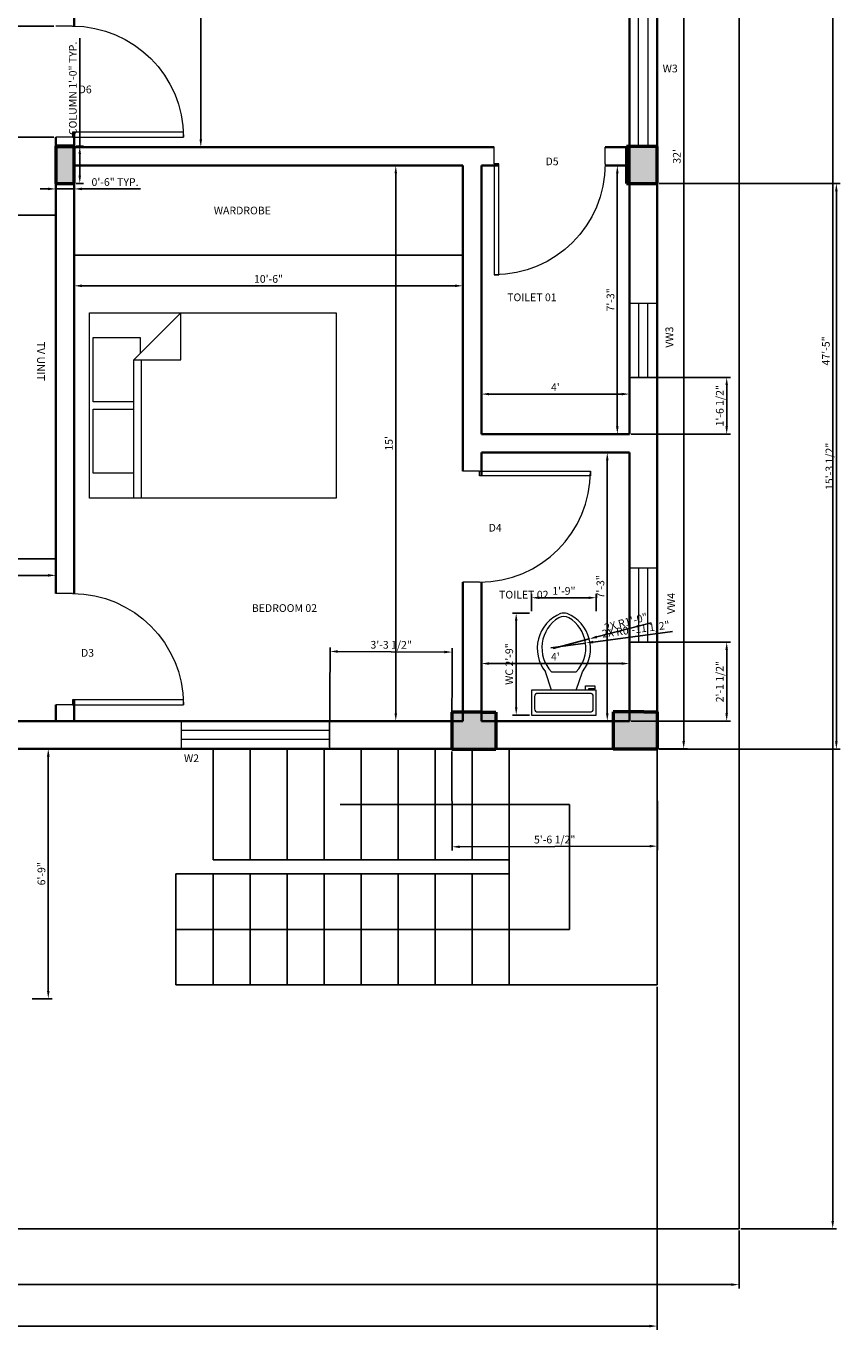
# Model space of a CAD drawing. Units: inches. Extents: x 2470 to 6338, y 1562 to 4199.
# Tile 2 of 5: x 2816 to 3080, y 1562 to 1985. Entities that reach past the tile are written whole.
import ezdxf

# ---------------------------------------------------------------- set-up
doc = ezdxf.new("R2010")
doc.units = ezdxf.units.IN
for name, color, linetype, lineweight in [('A-ANNO-DIMS', 2, 'Continuous', 18), ('A-ANNO-TEXT', 7, 'Continuous', 18), ('A-AREA-IDEN', 7, 'Continuous', 25), ('A-COLS', 1, 'Continuous', 50), ('A-DOOR', 4, 'Continuous', 18), ('A-FLOR-FIXT', 8, 'Continuous', 18), ('A-FLOR-STRS', 7, 'Continuous', 25), ('A-FURN', 8, 'Continuous', 18), ('A-FURN-FIXD', 8, 'Continuous', 25), ('A-GLAZ', 4, 'Continuous', 18), ('A-WALL', 7, 'Continuous', 35), ('C-PROP', 3, 'Continuous', 25)]:
    doc.layers.add(name, color=color, linetype=linetype, lineweight=lineweight)
doc.styles.get("Standard").update_dxf_attribs({"font": 'arial.ttf'})
doc.dimstyles.new('ISO-25', dxfattribs={"dimtxt": 2.5, "dimasz": 2.5, "dimexe": 1.25, "dimexo": 0.625, "dimtad": 1, "dimdec": 1, "dimlunit": 3, "dimtxsty": 'Standard', "dimcen": 2.5, "dimadec": 0, "dimazin": 0, "dimtfac": 1, "dimtdec": 1, "dimtmove": 0, "dimatfit": 3, "dimfxl": 1, "dimarcsym": 0})

# ---------------------------------------------------------------- blocks, each defined once
blk = doc.blocks.new('*U2')
for p, q in [((0, 0), (0, -6)), ((40, 0), (40, -6))]:
    blk.add_line(p, q)
blk.add_lwpolyline([(0, 0), (0, 40), (1.75, 40), (1.75, 0)], close=True)
blk.add_arc((0, 0), 40, 0, 90)
blk = doc.blocks.new('Toilet - top')
for p, q in [((9.5, -6), (9.5, -2)), ((-8, -8.5), (-8, -8)), ((-7, -8), (-7, -9.5)), ((-4, -8), (-6, -14)), ((4, -8), (6, -14)), ((-10, -8.5), (-8, -8.5)), ((-10, -9.5), (-10, -8.5)), ((-7, -9.5), (-10, -9.5)), ((4, -14), (-4, -14))]:
    blk.add_line(p, q)
blk.add_lwpolyline([(10.5, -8), (10.5, 0), (-10.5, 0), (-10.5, -8)], close=True)
for points in [[(-9.5, -2), (-9.5, -6)], [(8.5, -1), (-8.5, -1)], [(-8.5, -7), (8.5, -7)]]:
    blk.add_lwpolyline(points)
for centre, radius, start, end in [((-8.62, -1.88), 0.884, 81.8699, 188.1301), ((8.62, -1.88), 0.884, 351.8699, 98.1301), ((-8.62, -6.12), 0.884, 171.8699, 278.1301), ((8.62, -6.12), 0.884, 261.8699, 8.1301), ((3.52, -21.58), 12.17, 141.4691, 247.9714), ((4.2, -21.82), 11.33, 136.3677, 238.9468), ((-3.52, -21.58), 12.17, 292.0284, 38.5307), ((-4.2, -21.82), 11.33, 301.053, 43.6321), ((0, -27.88), 4, 245.7318, 294.2682), ((0, -29), 4, 254.8605, 285.1395)]:
    blk.add_arc(centre, radius, start, end)
blk = doc.blocks.new('Bed - Queen')
for p, q in [((0, -80.00003), (0, 0)), ((0, 0), (59.99999, 0)), ((59.99999, 0), (59.99999, -80.00003)), ((7.99999, -1.2), (28.79998, -1.2)), ((7.99999, -14.4), (7.99999, -1.2)), ((28.79998, -1.2), (28.79998, -14.4)), ((31.19999, -1.2), (51.99999, -1.2)), ((31.19999, -14.4), (31.19999, -1.2)), ((51.99999, -1.2), (51.99999, -16.4)), ((0, -14.4), (44.8, -14.4)), ((44.8, -16.8), (0, -16.8)), ((59.99999, -29.6), (44.8, -14.4)), ((44.8, -14.4), (44.8, -29.6)), ((51.99999, -16.4), (46.79936, -16.4)), ((44.8, -29.6), (59.99999, -29.6)), ((59.99999, -80.00003), (0, -80.00003))]:
    blk.add_line(p, q)
blk = doc.blocks.new('*D9')
at = {"layer": 'A-ANNO-DIMS', "color": 0, "lineweight": -2, "transparency": 16777216}
for p, q in [((3047.35, 2163.99), (3078.35, 2163.99)), ((3077.1, 2161.49), (3077.1, 1597.49)), ((3047.35, 1594.99), (3078.35, 1594.99))]:
    blk.add_line(p, q, dxfattribs=at)
at = {"layer": 'A-ANNO-DIMS', "color": 0, "lineweight": 100, "transparency": 16777216}
for points in [[(3076.68, 2161.49), (3077.51, 2161.49), (3077.1, 2163.99)], [(3076.68, 1597.49), (3077.51, 1597.49), (3077.1, 1594.99)]]:
    blk.add_solid(points, dxfattribs=at)
at = {"layer": 'Defpoints', "color": 0, "lineweight": 100, "transparency": 16777216}
for p in [(3046.72, 2163.99), (3046.72, 1594.99), (3077.1, 1594.99)]:
    blk.add_point(p, dxfattribs=at)
at = {"layer": 'A-ANNO-DIMS', "color": 0, "transparency": 16777216, "insert": (3075.2, 1879.49), "char_height": 2.5, "attachment_point": 5, "rotation": 90}
blk.add_mtext('47\'-5"', dxfattribs=at)
blk = doc.blocks.new('*D10')
at = {"layer": 'A-ANNO-DIMS', "color": 0, "lineweight": -2, "transparency": 16777216}
for p, q in [((2506.72, 1594.37), (2506.72, 1575.62)), ((3046.72, 1594.37), (3046.72, 1575.62)), ((2509.22, 1576.87), (3044.22, 1576.87))]:
    blk.add_line(p, q, dxfattribs=at)
at = {"layer": 'A-ANNO-DIMS', "color": 0, "lineweight": 100, "transparency": 16777216}
for points in [[(2509.22, 1577.29), (2509.22, 1576.46), (2506.72, 1576.87)], [(3044.22, 1577.29), (3044.22, 1576.46), (3046.72, 1576.87)]]:
    blk.add_solid(points, dxfattribs=at)
at = {"layer": 'Defpoints', "color": 0, "lineweight": 100, "transparency": 16777216}
for p in [(2506.72, 1594.99), (3046.72, 1594.99), (3046.72, 1576.87)]:
    blk.add_point(p, dxfattribs=at)
at = {"layer": 'A-ANNO-DIMS', "color": 0, "transparency": 16777216, "insert": (2776.72, 1578.77), "char_height": 2.5, "attachment_point": 5}
blk.add_mtext("45'", dxfattribs=at)
blk = doc.blocks.new('*D12')
at = {"layer": 'A-ANNO-DIMS', "color": 0, "lineweight": -2, "transparency": 16777216}
for p, q in [((3020.65, 2134.53), (3030.02, 2134.53)), ((3028.77, 2132.03), (3028.77, 1753.03)), ((3020.65, 1750.53), (3030.02, 1750.53))]:
    blk.add_line(p, q, dxfattribs=at)
at = {"layer": 'A-ANNO-DIMS', "color": 0, "lineweight": 100, "transparency": 16777216}
for points in [[(3028.36, 2132.03), (3029.19, 2132.03), (3028.77, 2134.53)], [(3028.36, 1753.03), (3029.19, 1753.03), (3028.77, 1750.53)]]:
    blk.add_solid(points, dxfattribs=at)
at = {"layer": 'Defpoints', "color": 0, "lineweight": 100, "transparency": 16777216}
for p in [(3020.03, 2134.53), (3020.03, 1750.53), (3028.77, 1750.53)]:
    blk.add_point(p, dxfattribs=at)
at = {"layer": 'A-ANNO-DIMS', "color": 0, "transparency": 16777216, "insert": (3026.87, 1942.53), "char_height": 2.5, "attachment_point": 5, "rotation": 90}
blk.add_mtext("32'", dxfattribs=at)
blk = doc.blocks.new('*D15')
at = {"layer": 'A-ANNO-DIMS', "color": 0, "lineweight": -2, "transparency": 16777216}
for p, q in [((2585.17, 1813.52), (2585.17, 1805.49)), ((2825.17, 1813.52), (2825.17, 1805.49)), ((2587.67, 1806.74), (2822.67, 1806.74))]:
    blk.add_line(p, q, dxfattribs=at)
at = {"layer": 'A-ANNO-DIMS', "color": 0, "lineweight": 100, "transparency": 16777216}
for points in [[(2587.67, 1807.16), (2587.67, 1806.32), (2585.17, 1806.74)], [(2822.67, 1807.16), (2822.67, 1806.32), (2825.17, 1806.74)]]:
    blk.add_solid(points, dxfattribs=at)
at = {"layer": 'Defpoints', "color": 0, "lineweight": 100, "transparency": 16777216}
for p in [(2585.17, 1814.14), (2825.17, 1814.14), (2825.17, 1806.74)]:
    blk.add_point(p, dxfattribs=at)
at = {"layer": 'A-ANNO-DIMS', "color": 0, "transparency": 16777216, "insert": (2705.17, 1808.64), "char_height": 2.5, "attachment_point": 5}
blk.add_mtext("20'", dxfattribs=at)
blk = doc.blocks.new('*D17')
at = {"layer": 'A-ANNO-DIMS', "color": 0, "lineweight": -2, "transparency": 16777216}
for p, q in [((2963.17, 1772.4), (2963.17, 1779.41)), ((3011.17, 1772.4), (3011.17, 1779.41)), ((2965.67, 1778.16), (3008.67, 1778.16))]:
    blk.add_line(p, q, dxfattribs=at)
at = {"layer": 'A-ANNO-DIMS', "color": 0, "lineweight": 100, "transparency": 16777216}
for points in [[(2965.67, 1778.58), (2965.67, 1777.75), (2963.17, 1778.16)], [(3008.67, 1778.58), (3008.67, 1777.75), (3011.17, 1778.16)]]:
    blk.add_solid(points, dxfattribs=at)
at = {"layer": 'Defpoints', "color": 0, "lineweight": 100, "transparency": 16777216}
for p in [(3011.17, 1778.16), (2963.17, 1771.78), (3011.17, 1771.78)]:
    blk.add_point(p, dxfattribs=at)
at = {"layer": 'A-ANNO-DIMS', "color": 0, "transparency": 16777216, "insert": (2987.17, 1780.04), "char_height": 2.5, "attachment_point": 5}
blk.add_mtext("4'", dxfattribs=at)
blk = doc.blocks.new('*D18')
at = {"layer": 'A-ANNO-DIMS', "color": 0, "lineweight": -2, "transparency": 16777216}
for p, q in [((3003.72, 1846.53), (3005.25, 1846.53)), ((3004, 1844.03), (3004, 1762.03)), ((3003.72, 1759.53), (3005.25, 1759.53))]:
    blk.add_line(p, q, dxfattribs=at)
at = {"layer": 'A-ANNO-DIMS', "color": 0, "lineweight": 100, "transparency": 16777216}
for points in [[(3003.58, 1844.03), (3004.41, 1844.03), (3004, 1846.53)], [(3003.58, 1762.03), (3004.41, 1762.03), (3004, 1759.53)]]:
    blk.add_solid(points, dxfattribs=at)
at = {"layer": 'Defpoints', "color": 0, "lineweight": 100, "transparency": 16777216}
for p in [(3003.1, 1846.53), (3003.1, 1759.53), (3004, 1759.53)]:
    blk.add_point(p, dxfattribs=at)
at = {"layer": 'A-ANNO-DIMS', "color": 0, "transparency": 16777216, "insert": (3002.1, 1803.03), "char_height": 2.5, "attachment_point": 5, "rotation": 90}
blk.add_mtext('7\'-3"', dxfattribs=at)
blk = doc.blocks.new('*D19')
at = {"layer": 'A-ANNO-DIMS', "color": 0, "lineweight": -2, "transparency": 16777216}
for p, q in [((2963.17, 1870.28), (2963.17, 1864.24)), ((3011.17, 1870.27), (3011.17, 1864.24)), ((2965.67, 1865.49), (3008.67, 1865.49))]:
    blk.add_line(p, q, dxfattribs=at)
at = {"layer": 'A-ANNO-DIMS', "color": 0, "lineweight": 100, "transparency": 16777216}
for points in [[(2965.67, 1865.91), (2965.67, 1865.08), (2963.17, 1865.49)], [(3008.67, 1865.91), (3008.67, 1865.08), (3011.17, 1865.49)]]:
    blk.add_solid(points, dxfattribs=at)
at = {"layer": 'Defpoints', "color": 0, "lineweight": 100, "transparency": 16777216}
for p in [(2963.17, 1870.9), (3011.17, 1870.9), (3011.17, 1865.49)]:
    blk.add_point(p, dxfattribs=at)
at = {"layer": 'A-ANNO-DIMS', "color": 0, "transparency": 16777216, "insert": (2987.17, 1867.37), "char_height": 2.5, "attachment_point": 5}
blk.add_mtext("4'", dxfattribs=at)
blk = doc.blocks.new('*D20')
at = {"layer": 'A-ANNO-DIMS', "color": 0, "lineweight": -2, "transparency": 16777216}
for p, q in [((3007.26, 1937.03), (3007.26, 1855.03)), ((3007.86, 1939.53), (3008.51, 1939.53)), ((3007.86, 1852.53), (3008.51, 1852.53))]:
    blk.add_line(p, q, dxfattribs=at)
at = {"layer": 'A-ANNO-DIMS', "color": 0, "lineweight": 100, "transparency": 16777216}
for points in [[(3006.84, 1937.03), (3007.68, 1937.03), (3007.26, 1939.53)], [(3006.84, 1855.03), (3007.68, 1855.03), (3007.26, 1852.53)]]:
    blk.add_solid(points, dxfattribs=at)
at = {"layer": 'Defpoints', "color": 0, "lineweight": 100, "transparency": 16777216}
for p in [(3007.23, 1939.53), (3007.23, 1852.53), (3007.26, 1852.53)]:
    blk.add_point(p, dxfattribs=at)
at = {"layer": 'A-ANNO-DIMS', "color": 0, "transparency": 16777216, "insert": (3005.36, 1896.03), "char_height": 2.5, "attachment_point": 5, "rotation": 90}
blk.add_mtext('7\'-3"', dxfattribs=at)
blk = doc.blocks.new('*D21')
at = {"layer": 'A-ANNO-DIMS', "color": 0, "lineweight": -2, "transparency": 16777216}
for p, q in [((2831.17, 1901.89), (2831.17, 1899.33)), ((2957.17, 1901.89), (2957.17, 1899.33)), ((2833.67, 1900.58), (2954.67, 1900.58))]:
    blk.add_line(p, q, dxfattribs=at)
at = {"layer": 'A-ANNO-DIMS', "color": 0, "lineweight": 100, "transparency": 16777216}
for points in [[(2833.67, 1901), (2833.67, 1900.17), (2831.17, 1900.58)], [(2954.67, 1901), (2954.67, 1900.17), (2957.17, 1900.58)]]:
    blk.add_solid(points, dxfattribs=at)
at = {"layer": 'Defpoints', "color": 0, "lineweight": 100, "transparency": 16777216}
for p in [(2831.17, 1902.52), (2957.17, 1902.52), (2957.17, 1900.58)]:
    blk.add_point(p, dxfattribs=at)
at = {"layer": 'A-ANNO-DIMS', "color": 0, "transparency": 16777216, "insert": (2894.17, 1902.49), "char_height": 2.5, "attachment_point": 5}
blk.add_mtext('10\'-6"', dxfattribs=at)
blk = doc.blocks.new('*D22')
at = {"layer": 'A-ANNO-DIMS', "color": 0, "lineweight": -2, "transparency": 16777216}
for p, q in [((2925.41, 1939.53), (2936.67, 1939.53)), ((2935.42, 1937.03), (2935.42, 1762.03)), ((2925.41, 1759.53), (2936.67, 1759.53))]:
    blk.add_line(p, q, dxfattribs=at)
at = {"layer": 'A-ANNO-DIMS', "color": 0, "lineweight": 100, "transparency": 16777216}
for points in [[(2935.01, 1937.03), (2935.84, 1937.03), (2935.42, 1939.53)], [(2935.01, 1762.03), (2935.84, 1762.03), (2935.42, 1759.53)]]:
    blk.add_solid(points, dxfattribs=at)
at = {"layer": 'Defpoints', "color": 0, "lineweight": 100, "transparency": 16777216}
for p in [(2924.78, 1939.53), (2924.78, 1759.53), (2935.42, 1759.53)]:
    blk.add_point(p, dxfattribs=at)
at = {"layer": 'A-ANNO-DIMS', "color": 0, "transparency": 16777216, "insert": (2933.52, 1849.53), "char_height": 2.5, "attachment_point": 5, "rotation": 90}
blk.add_mtext("15'", dxfattribs=at)
blk = doc.blocks.new('*D30')
at = {"layer": 'A-ANNO-DIMS', "color": 0, "lineweight": -2, "transparency": 16777216}
for p, q in [((2859.5, 2125.53), (2873.46, 2125.53)), ((2872.21, 2123.03), (2872.21, 1948.03)), ((2867.05, 1945.53), (2873.46, 1945.53))]:
    blk.add_line(p, q, dxfattribs=at)
at = {"layer": 'A-ANNO-DIMS', "color": 0, "lineweight": 100, "transparency": 16777216}
for points in [[(2871.79, 2123.03), (2872.62, 2123.03), (2872.21, 2125.53)], [(2871.79, 1948.03), (2872.62, 1948.03), (2872.21, 1945.53)]]:
    blk.add_solid(points, dxfattribs=at)
at = {"layer": 'Defpoints', "color": 0, "lineweight": 100, "transparency": 16777216}
for p in [(2858.88, 2125.53), (2866.42, 1945.53), (2872.21, 1945.53)]:
    blk.add_point(p, dxfattribs=at)
at = {"layer": 'A-ANNO-DIMS', "color": 0, "transparency": 16777216, "insert": (2870.31, 2035.53), "char_height": 2.5, "attachment_point": 5, "rotation": 90}
blk.add_mtext("15'", dxfattribs=at)
blk = doc.blocks.new('*D31')
at = {"layer": 'A-ANNO-DIMS', "color": 0, "lineweight": -2, "transparency": 16777216}
for p, q in [((2817.49, 1750.53), (2824.01, 1750.53)), ((2822.76, 1748.03), (2822.76, 1672.03)), ((2817.49, 1669.53), (2824.01, 1669.53))]:
    blk.add_line(p, q, dxfattribs=at)
at = {"layer": 'A-ANNO-DIMS', "color": 0, "lineweight": 100, "transparency": 16777216}
for points in [[(2822.34, 1748.03), (2823.18, 1748.03), (2822.76, 1750.53)], [(2822.34, 1672.03), (2823.18, 1672.03), (2822.76, 1669.53)]]:
    blk.add_solid(points, dxfattribs=at)
at = {"layer": 'Defpoints', "color": 0, "lineweight": 100, "transparency": 16777216}
for p in [(2816.87, 1750.53), (2816.87, 1669.53), (2822.76, 1669.53)]:
    blk.add_point(p, dxfattribs=at)
at = {"layer": 'A-ANNO-DIMS', "color": 0, "transparency": 16777216, "insert": (2820.86, 1710.03), "char_height": 2.5, "attachment_point": 5, "rotation": 90}
blk.add_mtext('6\'-9"', dxfattribs=at)
blk = doc.blocks.new('WIN-48IN')
for p, q in [((0, 9), (48, 9)), ((0, 0), (0, 9)), ((48, 9), (48, 0)), ((0, 6), (48, 6)), ((48, 3), (0, 3)), ((48, 0), (0, 0))]:
    blk.add_line(p, q)
blk = doc.blocks.new('VENT-WIN-24IN')
for p, q in [((9, 24), (0, 24)), ((0, 24), (0, 0)), ((3, 24), (3, 0)), ((6, 0), (6, 24)), ((9, 0), (9, 24)), ((0, 0), (9, 0))]:
    blk.add_line(p, q)
blk = doc.blocks.new('COL-6X12')
h = blk.add_hatch(color=256)
h.dxf.hatch_style = 1
h.paths.add_polyline_path([(6, 12), (0, 12), (0, 0), (6, 0)])
for p, q in [((6, 12), (0, 12)), ((0, 12), (0, 0)), ((6, 0), (6, 12)), ((0, 0), (6, 0))]:
    blk.add_line(p, q)
blk = doc.blocks.new('COL-10X12')
h = blk.add_hatch(color=256)
h.dxf.hatch_style = 1
h.paths.add_polyline_path([(10, 12), (0, 12), (0, 0), (10, 0)])
for p, q in [((10, 12), (0, 12)), ((0, 12), (0, 0)), ((10, 0), (10, 12)), ((0, 0), (10, 0))]:
    blk.add_line(p, q)
blk = doc.blocks.new('COL-RECT-LARGE')
h = blk.add_hatch(color=256)
h.dxf.hatch_style = 1
h.paths.add_polyline_path([(14.33, 12.11), (10, 12.11), (0, 12.11), (0, 0), (10, 0), (14.33, 0)])
for p, q in [((10, 12.11), (0, 12.11)), ((0, 12.11), (0, 0)), ((10, 12.11), (14.33, 12.11)), ((14.33, 12.11), (14.33, 0)), ((10, 0), (0, 0)), ((14.33, 0), (10, 0))]:
    blk.add_line(p, q)
blk = doc.blocks.new('*D48')
at = {"layer": 'A-ANNO-DIMS', "color": 0, "lineweight": -2, "transparency": 16777216}
for p, q in [((2832.97, 1945.79), (2832.97, 1980.85)), ((2831.79, 1945.79), (2834.22, 1945.79)), ((2832.97, 1936.29), (2832.97, 1943.29)), ((2831.79, 1933.79), (2834.22, 1933.79))]:
    blk.add_line(p, q, dxfattribs=at)
at = {"layer": 'A-ANNO-DIMS', "color": 0, "lineweight": 100, "transparency": 16777216}
for points in [[(2832.55, 1943.29), (2833.38, 1943.29), (2832.97, 1945.79)], [(2832.55, 1936.29), (2833.38, 1936.29), (2832.97, 1933.79)]]:
    blk.add_solid(points, dxfattribs=at)
at = {"layer": 'Defpoints', "color": 0, "lineweight": 100, "transparency": 16777216}
for p in [(2831.17, 1945.79), (2832.97, 1945.79), (2831.17, 1933.79)]:
    blk.add_point(p, dxfattribs=at)
at = {"layer": 'A-ANNO-DIMS', "color": 0, "transparency": 16777216, "insert": (2831.05, 1964.57), "char_height": 2.5, "attachment_point": 5, "rotation": 90}
blk.add_mtext('COLUMN 1\'-0" TYP.', dxfattribs=at)
blk = doc.blocks.new('*D49')
at = {"layer": 'A-ANNO-DIMS', "color": 0, "lineweight": -2, "transparency": 16777216}
for p, q in [((2822.67, 1931.99), (2820.17, 1931.99)), ((2825.17, 1933.16), (2825.17, 1930.74)), ((2825.17, 1931.99), (2831.17, 1931.99)), ((2831.17, 1933.16), (2831.17, 1930.74)), ((2833.67, 1931.99), (2852.66, 1931.99))]:
    blk.add_line(p, q, dxfattribs=at)
at = {"layer": 'A-ANNO-DIMS', "color": 0, "lineweight": 100, "transparency": 16777216}
for points in [[(2822.67, 1932.41), (2822.67, 1931.57), (2825.17, 1931.99)], [(2833.67, 1932.41), (2833.67, 1931.57), (2831.17, 1931.99)]]:
    blk.add_solid(points, dxfattribs=at)
at = {"layer": 'Defpoints', "color": 0, "lineweight": 100, "transparency": 16777216}
for p in [(2825.17, 1933.79), (2831.17, 1933.79), (2831.17, 1931.99)]:
    blk.add_point(p, dxfattribs=at)
at = {"layer": 'A-ANNO-DIMS', "color": 0, "transparency": 16777216, "insert": (2844.41, 1933.89), "char_height": 2.5, "attachment_point": 5}
blk.add_mtext('0\'-6" TYP.', dxfattribs=at)
blk = doc.blocks.new('*D56')
at = {"layer": 'A-ANNO-DIMS', "color": 0, "lineweight": -2, "transparency": 16777216}
for p, q in [((2978.8, 1794.53), (2973.22, 1794.53)), ((2974.47, 1792.03), (2974.47, 1763.98)), ((2978.8, 1761.48), (2973.22, 1761.48))]:
    blk.add_line(p, q, dxfattribs=at)
at = {"layer": 'A-ANNO-DIMS', "color": 0, "lineweight": 100, "transparency": 16777216}
for points in [[(2974.06, 1792.03), (2974.89, 1792.03), (2974.47, 1794.53)], [(2974.06, 1763.98), (2974.89, 1763.98), (2974.47, 1761.48)]]:
    blk.add_solid(points, dxfattribs=at)
at = {"layer": 'Defpoints', "color": 0, "lineweight": 100, "transparency": 16777216}
for p in [(2979.43, 1794.53), (2974.47, 1761.48), (2979.43, 1761.48)]:
    blk.add_point(p, dxfattribs=at)
at = {"layer": 'A-ANNO-DIMS', "color": 0, "transparency": 16777216, "insert": (2972.55, 1778), "char_height": 2.5, "attachment_point": 5, "rotation": 90}
blk.add_mtext('WC 2\'-9"', dxfattribs=at)
blk = doc.blocks.new('*D57')
at = {"layer": 'A-ANNO-DIMS', "color": 0, "lineweight": -2, "transparency": 16777216}
for p, q in [((2979.43, 1795.15), (2979.43, 1800.73)), ((3000.43, 1795.15), (3000.43, 1800.73)), ((2997.93, 1799.48), (2981.93, 1799.48))]:
    blk.add_line(p, q, dxfattribs=at)
at = {"layer": 'A-ANNO-DIMS', "color": 0, "lineweight": 100, "transparency": 16777216}
for points in [[(2981.93, 1799.9), (2981.93, 1799.07), (2979.43, 1799.48)], [(2997.93, 1799.9), (2997.93, 1799.07), (3000.43, 1799.48)]]:
    blk.add_solid(points, dxfattribs=at)
at = {"layer": 'Defpoints', "color": 0, "lineweight": 100, "transparency": 16777216}
for p in [(2979.43, 1799.48), (2979.43, 1794.53), (3000.43, 1794.53)]:
    blk.add_point(p, dxfattribs=at)
at = {"layer": 'A-ANNO-DIMS', "color": 0, "transparency": 16777216, "insert": (2989.93, 1801.38), "char_height": 2.5, "attachment_point": 5}
blk.add_mtext('1\'-9"', dxfattribs=at)
blk = doc.blocks.new('*D58')
at = {"layer": 'A-ANNO-DIMS', "color": 0, "lineweight": -2, "transparency": 16777216}
for p, q in [((3020.17, 1673.39), (3020.17, 1562.19)), ((2528.17, 1668.91), (2528.17, 1562.19)), ((2530.67, 1563.44), (3017.67, 1563.44))]:
    blk.add_line(p, q, dxfattribs=at)
at = {"layer": 'A-ANNO-DIMS', "color": 0, "lineweight": 100, "transparency": 16777216}
for points in [[(2530.67, 1563.86), (2530.67, 1563.02), (2528.17, 1563.44)], [(3017.67, 1563.86), (3017.67, 1563.02), (3020.17, 1563.44)]]:
    blk.add_solid(points, dxfattribs=at)
at = {"layer": 'Defpoints', "color": 0, "lineweight": 100, "transparency": 16777216}
for p in [(3020.17, 1674.02), (2528.17, 1669.53), (3020.17, 1563.44)]:
    blk.add_point(p, dxfattribs=at)
at = {"layer": 'A-ANNO-DIMS', "color": 0, "transparency": 16777216, "insert": (2774.17, 1565.34), "char_height": 2.5, "attachment_point": 5}
blk.add_mtext('41\'-0"', dxfattribs=at)
blk = doc.blocks.new('*D63')
at = {"layer": 'A-ANNO-DIMS', "color": 0, "lineweight": -2, "transparency": 16777216}
for p, q in [((2953.56, 1749.7), (2953.66, 1717.53)), ((3020.17, 1749.91), (3020.27, 1717.73)), ((3017.76, 1718.98), (2956.15, 1718.79))]:
    blk.add_line(p, q, dxfattribs=at)
at = {"layer": 'A-ANNO-DIMS', "color": 0, "lineweight": 100, "transparency": 16777216}
for points in [[(2956.15, 1719.2), (2956.15, 1718.37), (2953.65, 1718.78)], [(3017.76, 1719.39), (3017.77, 1718.56), (3020.26, 1718.98)]]:
    blk.add_solid(points, dxfattribs=at)
at = {"layer": 'Defpoints', "color": 0, "lineweight": 100, "transparency": 16777216}
for p in [(2953.56, 1750.33), (3020.17, 1750.53), (2953.65, 1718.78)]:
    blk.add_point(p, dxfattribs=at)
at = {"layer": 'A-ANNO-DIMS', "color": 0, "transparency": 16777216, "insert": (2986.95, 1720.8), "char_height": 2.5, "attachment_point": 5, "rotation": 0.1759}
blk.add_mtext('5\'-6 1/2"', dxfattribs=at)
blk = doc.blocks.new('*D64')
at = {"layer": 'A-ANNO-DIMS', "color": 0, "lineweight": -2, "transparency": 16777216}
for p, q in [((3020.85, 1933.73), (3079.52, 1933.73)), ((3078.27, 1752.93), (3078.27, 1931.23)), ((3020.83, 1750.43), (3079.52, 1750.43))]:
    blk.add_line(p, q, dxfattribs=at)
at = {"layer": 'A-ANNO-DIMS', "color": 0, "lineweight": 100, "transparency": 16777216}
for points in [[(3077.86, 1931.23), (3078.69, 1931.23), (3078.27, 1933.73)], [(3077.86, 1752.93), (3078.69, 1752.93), (3078.27, 1750.43)]]:
    blk.add_solid(points, dxfattribs=at)
at = {"layer": 'Defpoints', "color": 0, "lineweight": 100, "transparency": 16777216}
for p in [(3020.23, 1933.73), (3078.27, 1933.73), (3020.2, 1750.43)]:
    blk.add_point(p, dxfattribs=at)
at = {"layer": 'A-ANNO-DIMS', "color": 0, "transparency": 16777216, "insert": (3076.35, 1842.08), "char_height": 2.5, "attachment_point": 5, "rotation": 90}
blk.add_mtext('15\'-3 1/2"', dxfattribs=at)
blk = doc.blocks.new('*D69')
at = {"layer": 'A-ANNO-DIMS', "color": 0, "lineweight": -2, "transparency": 16777216}
for p, q in [((2824.54, 1984.76), (2792.37, 1984.76)), ((2793.62, 1951.26), (2793.62, 1982.26)), ((2824.54, 1948.76), (2792.37, 1948.76))]:
    blk.add_line(p, q, dxfattribs=at)
at = {"layer": 'A-ANNO-DIMS', "color": 0, "lineweight": 100, "transparency": 16777216}
for points in [[(2793.2, 1982.26), (2794.03, 1982.26), (2793.62, 1984.76)], [(2793.2, 1951.26), (2794.03, 1951.26), (2793.62, 1948.76)]]:
    blk.add_solid(points, dxfattribs=at)
at = {"layer": 'Defpoints', "color": 0, "lineweight": 100, "transparency": 16777216}
for p in [(2793.62, 1984.76), (2825.17, 1984.76), (2825.17, 1948.76)]:
    blk.add_point(p, dxfattribs=at)
at = {"layer": 'A-ANNO-DIMS', "color": 0, "transparency": 16777216, "insert": (2791.72, 1966.76), "char_height": 2.5, "attachment_point": 5, "rotation": 90}
blk.add_mtext('3\'-0"', dxfattribs=at)
blk = doc.blocks.new('*D74')
at = {"layer": 'A-ANNO-DIMS', "color": 0, "lineweight": -2, "transparency": 16777216}
for p, q in [((2913.96, 1751.16), (2914.12, 1783.33)), ((2916.62, 1782.07), (2951.22, 1781.89)), ((2953.56, 1750.95), (2953.73, 1783.13))]:
    blk.add_line(p, q, dxfattribs=at)
at = {"layer": 'A-ANNO-DIMS', "color": 0, "lineweight": 100, "transparency": 16777216}
for points in [[(2916.62, 1782.49), (2916.62, 1781.65), (2914.12, 1782.08)], [(2951.22, 1782.31), (2951.22, 1781.48), (2953.72, 1781.88)]]:
    blk.add_solid(points, dxfattribs=at)
at = {"layer": 'Defpoints', "color": 0, "lineweight": 100, "transparency": 16777216}
for p in [(2953.72, 1781.88), (2913.95, 1750.53), (2953.56, 1750.33)]:
    blk.add_point(p, dxfattribs=at)
at = {"layer": 'A-ANNO-DIMS', "color": 0, "transparency": 16777216, "insert": (2933.93, 1783.9), "char_height": 2.5, "attachment_point": 5, "rotation": 359.7042}
blk.add_mtext('3\'-3 1/2"', dxfattribs=at)
blk = doc.blocks.new('*D78')
at = {"layer": 'A-ANNO-DIMS', "color": 0, "lineweight": -2, "transparency": 16777216}
for p, q in [((3011.79, 1785.06), (3043.97, 1785.06)), ((3042.72, 1782.56), (3042.72, 1762.03)), ((3011.79, 1759.53), (3043.97, 1759.53))]:
    blk.add_line(p, q, dxfattribs=at)
at = {"layer": 'A-ANNO-DIMS', "color": 0, "lineweight": 100, "transparency": 16777216}
for points in [[(3042.3, 1782.56), (3043.13, 1782.56), (3042.72, 1785.06)], [(3042.3, 1762.03), (3043.13, 1762.03), (3042.72, 1759.53)]]:
    blk.add_solid(points, dxfattribs=at)
at = {"layer": 'Defpoints', "color": 0, "lineweight": 100, "transparency": 16777216}
for p in [(3011.17, 1785.06), (3011.17, 1759.53), (3042.72, 1759.53)]:
    blk.add_point(p, dxfattribs=at)
at = {"layer": 'A-ANNO-DIMS', "color": 0, "transparency": 16777216, "insert": (3040.8, 1772.3), "char_height": 2.5, "attachment_point": 5, "rotation": 90}
blk.add_mtext('2\'-1 1/2"', dxfattribs=at)
blk = doc.blocks.new('*D79')
at = {"layer": 'A-ANNO-DIMS', "color": 0, "lineweight": -2, "transparency": 16777216}
for p, q in [((3011.79, 1870.9), (3043.97, 1870.9)), ((3042.72, 1868.4), (3042.72, 1855.03)), ((3011.79, 1852.53), (3043.97, 1852.53))]:
    blk.add_line(p, q, dxfattribs=at)
at = {"layer": 'A-ANNO-DIMS', "color": 0, "lineweight": 100, "transparency": 16777216}
for points in [[(3042.3, 1868.4), (3043.13, 1868.4), (3042.72, 1870.9)], [(3042.3, 1855.03), (3043.13, 1855.03), (3042.72, 1852.53)]]:
    blk.add_solid(points, dxfattribs=at)
at = {"layer": 'Defpoints', "color": 0, "lineweight": 100, "transparency": 16777216}
for p in [(3011.17, 1870.9), (3011.17, 1852.53), (3042.72, 1852.53)]:
    blk.add_point(p, dxfattribs=at)
at = {"layer": 'A-ANNO-DIMS', "color": 0, "transparency": 16777216, "insert": (3040.8, 1861.72), "char_height": 2.5, "attachment_point": 5, "rotation": 90}
blk.add_mtext('1\'-6 1/2"', dxfattribs=at)
blk = doc.blocks.new('*D80')
at = {"layer": 'A-ANNO-DIMS', "color": 0, "lineweight": -2, "transparency": 16777216}
for p, q in [((3018.2, 1791.41), (3000.6, 1786.79)), ((2986.41, 1783.06), (2998.18, 1786.15))]:
    blk.add_line(p, q, dxfattribs=at)
at = {"layer": 'A-ANNO-DIMS', "color": 0, "lineweight": 100, "transparency": 16777216}
blk.add_solid([(3000.49, 1787.19), (3000.7, 1786.39), (2998.18, 1786.15)], dxfattribs=at)
at = {"layer": 'Defpoints', "color": 0, "lineweight": 100, "transparency": 16777216}
for p in [(2998.18, 1786.15), (2986.41, 1783.06)]:
    blk.add_point(p, dxfattribs=at)
at = {"layer": 'A-ANNO-DIMS', "color": 0, "transparency": 16777216, "insert": (3010.13, 1791.26), "char_height": 2.5, "attachment_point": 5, "rotation": 14.7223}
blk.add_mtext('2X R1\'-0"', dxfattribs=at)
blk = doc.blocks.new('*D81')
at = {"layer": 'A-ANNO-DIMS', "color": 0, "lineweight": -2, "transparency": 16777216}
for p, q in [((3025.17, 1788.6), (2999.43, 1785.14)), ((2985.73, 1783.3), (2996.96, 1784.81))]:
    blk.add_line(p, q, dxfattribs=at)
at = {"layer": 'A-ANNO-DIMS', "color": 0, "lineweight": 100, "transparency": 16777216}
blk.add_solid([(2999.38, 1785.55), (2999.49, 1784.73), (2996.96, 1784.81)], dxfattribs=at)
at = {"layer": 'Defpoints', "color": 0, "lineweight": 100, "transparency": 16777216}
for p in [(2985.73, 1783.3), (2996.96, 1784.81)]:
    blk.add_point(p, dxfattribs=at)
at = {"layer": 'A-ANNO-DIMS', "color": 0, "transparency": 16777216, "insert": (3013.29, 1788.94), "char_height": 2.5, "attachment_point": 5, "rotation": 7.6578}
blk.add_mtext('2X R0\'-11 1/2"', dxfattribs=at)

msp = doc.modelspace()

# ---------------------------------------------------------------- linework, layer by layer
at = {"layer": 'A-FLOR-STRS'}
for p, q in [((2876.17, 1750.53), (2876.17, 1714.53)), ((2888.17, 1750.53), (2888.17, 1714.53)), ((2900.17, 1750.53), (2900.17, 1714.53)), ((2912.17, 1750.53), (2912.17, 1714.53)), ((2924.17, 1750.53), (2924.17, 1714.53)), ((2936.17, 1750.53), (2936.17, 1714.53)), ((2948.17, 1750.53), (2948.17, 1714.53)), ((2960.17, 1750.53), (2960.17, 1714.53)), ((2972.17, 1750.53), (2972.17, 1674.02)), ((3020.17, 1750.53), (3020.17, 1674.02)), ((2972.17, 1732.53), (2917.43, 1732.53)), ((2972.17, 1732.53), (2991.72, 1732.53)), ((2991.72, 1692.02), (2991.72, 1732.53)), ((2972.17, 1714.53), (2876.17, 1714.53)), ((2864.17, 1710.02), (2864.17, 1674.02)), ((2972.17, 1710.02), (2864.17, 1710.02)), ((2876.17, 1710.02), (2876.17, 1674.02)), ((2888.17, 1710.02), (2888.17, 1674.02)), ((2900.17, 1710.02), (2900.17, 1674.02)), ((2912.17, 1710.02), (2912.17, 1674.02)), ((2924.17, 1710.02), (2924.17, 1674.02)), ((2936.17, 1710.02), (2936.17, 1674.02)), ((2948.17, 1710.02), (2948.17, 1674.02)), ((2960.17, 1710.02), (2960.17, 1674.02)), ((2864.17, 1692.02), (2991.72, 1692.02)), ((3020.17, 1674.02), (2864.17, 1674.02))]:
    msp.add_line(p, q, dxfattribs=at)
at = {"layer": 'A-FURN-FIXD'}
msp.add_line((2831.17, 1910.47), (2957.17, 1910.47), dxfattribs=at)
msp.add_lwpolyline([(2825.17, 1923.49), (2811.05, 1923.49), (2811.05, 1812.14), (2825.17, 1812.14)], close=True, dxfattribs=at)
at = {"layer": 'A-WALL'}
for p, q in [((3020.17, 2134.53), (3020.17, 1750.53)), ((2831.17, 2125.53), (2831.17, 1984.76)), ((3011.17, 2125.53), (3011.17, 1852.53)), ((2825.17, 1948.76), (2825.17, 1800.83)), ((2831.17, 1950.34), (2831.17, 1945.53)), ((2831.17, 1945.53), (2825.17, 1945.53)), ((2831.17, 1945.53), (2967.3, 1945.53)), ((3003.3, 1945.53), (3011.17, 1945.53)), ((2831.17, 1939.53), (2957.17, 1939.53)), ((2831.17, 1939.53), (2831.17, 1800.82)), ((2957.17, 1939.53), (2957.17, 1840.54)), ((2963.17, 1939.53), (2963.17, 1852.53)), ((2963.17, 1939.53), (2968.87, 1939.53)), ((3003.29, 1939.53), (3011.17, 1939.53)), ((3011.17, 1852.53), (2963.17, 1852.53)), ((3011.17, 1846.53), (2963.17, 1846.53)), ((2963.17, 1846.53), (2963.17, 1838.97)), ((3011.17, 1846.53), (3011.17, 1759.53)), ((2957.17, 1804.54), (2957.17, 1759.53)), ((2963.17, 1804.55), (2963.17, 1759.53)), ((2831.17, 1766.4), (2831.17, 1759.53)), ((2825.17, 1764.83), (2825.17, 1759.53)), ((2957.17, 1759.53), (2797.73, 1759.53)), ((3011.17, 1759.53), (2963.17, 1759.53)), ((3020.17, 1750.53), (2576.17, 1750.53))]:
    msp.add_line(p, q, dxfattribs=at)
at = {"layer": 'C-PROP'}
for p, q in [((3046.72, 2163.99), (3046.72, 1594.99)), ((3046.72, 1594.99), (2506.72, 1594.99))]:
    msp.add_line(p, q, dxfattribs=at)

# ---------------------------------------------------------------- block references
at = {"layer": 'A-COLS'}
for name, p in [('COL-6X12', (2825.17, 1933.79)), ('COL-10X12', (3010.23, 1933.73)), ('COL-RECT-LARGE', (2953.56, 1750.33)), ('COL-RECT-LARGE', (3005.88, 1750.43))]:
    msp.add_blockref(name, p, dxfattribs=at)
at = {"layer": 'A-DOOR', "yscale": 0.9, "zscale": 0.9}
for p, xscale, rotation in [((2830.57, 1948.76), -0.9, 270), ((2967.3, 1940.13), -0.9, 180), ((2962.57, 1840.54), 0.9, 270), ((2830.57, 1764.83), -0.9, 270)]:
    msp.add_blockref('*U2', p, dxfattribs=dict(at, xscale=xscale, rotation=rotation))
at = {"layer": 'A-FLOR-FIXT', "rotation": 180}
msp.add_blockref('Toilet - top', (2989.93, 1761.48), dxfattribs=at)
at = {"layer": 'A-FURN', "rotation": 90}
msp.add_blockref('Bed - Queen', (2836.11, 1831.81), dxfattribs=at)
at = {"layer": 'A-GLAZ', "rotation": 89.9999999999996}
msp.add_blockref('WIN-48IN', (3020.17, 1945.73), dxfattribs=at)
at = {"layer": 'A-GLAZ'}
for name, p in [('VENT-WIN-24IN', (3011.17, 1870.9)), ('VENT-WIN-24IN', (3011.17, 1785.06)), ('WIN-48IN', (2865.95, 1750.53))]:
    msp.add_blockref(name, p, dxfattribs=at)

# ---------------------------------------------------------------- texts
at = {"layer": 'A-ANNO-TEXT', "char_height": 2.5, "attachment_point": 1}
for s, width, insert in [('W3', 4.502, (3021.96, 1972.26)), ('D6', 11.6764, (2832.6, 1965.49)), ('D5', 13.1773, (2983.98, 1942.16)), ('WARDROBE', 44.6529, (2876.43, 1926.24)), ('D4', 15.7726, (2965.54, 1823.42)), ('D3', 10.3463, (2833.37, 1782.88)), ('W2', 6.8755, (2866.76, 1748.71))]:
    msp.add_mtext_dynamic_manual_height_columns(s, width=width, gutter_width=12.5, heights=[0], dxfattribs=dict(at, insert=insert))
for s, width, insert, rotation in [('VW3', 11.5293, (3022.88, 1880.52), 90), ('TV UNIT', 25.1044, (2821.65, 1882.45), 270), ('VW4', 15.1929, (3023.45, 1794.21), 90)]:
    msp.add_mtext_dynamic_manual_height_columns(s, width=width, gutter_width=12.5, heights=[0], dxfattribs=dict(at, insert=insert, rotation=rotation))
at = {"layer": 'A-AREA-IDEN', "char_height": 2.5, "attachment_point": 1}
for s, width, insert in [('TOILET 01', 24.38, (2971.55, 1898.1)), ('TOILET 02', 23.0446, (2968.92, 1801.73)), ('BEDROOM 02', 44.793, (2888.76, 1797.39))]:
    msp.add_mtext_dynamic_manual_height_columns(s, width=width, gutter_width=12.5, heights=[0], dxfattribs=dict(at, insert=insert))

# ---------------------------------------------------------------- dimensions: what is measured, and where the dimension line sits
at = {"layer": 'A-ANNO-DIMS'}
for base, p1, p2, angle, override, picture, middle in [((3077.1, 1594.99), (3046.72, 2163.99), (3046.72, 1594.99), 90, {"dimclrd": 0, "dimclre": 0, "dimclrt": 0}, '*D9', (3075.2, 1879.49)), ((3028.77, 1750.53), (3020.03, 2134.53), (3020.03, 1750.53), 90, {"dimclrd": 0, "dimclre": 0, "dimclrt": 0}, '*D12', (3026.87, 1942.53)), ((2872.21, 1945.53), (2858.88, 2125.53), (2866.42, 1945.53), 90, {"dimclrd": 0, "dimclre": 0, "dimclrt": 0}, '*D30', (2870.31, 2035.53)), ((2793.62, 1984.76), (2825.17, 1948.76), (2825.17, 1984.76), 90, {"dimdec": 1, "dimlfac": 1, "dimrnd": 0, "dimzin": 1, "dimdsep": 46, "dimlunit": 4, "dimfrac": 2}, '*D69', (2791.72, 1966.76)), ((2935.42, 1759.53), (2924.78, 1939.53), (2924.78, 1759.53), 90, {"dimclrd": 0, "dimclre": 0, "dimclrt": 0}, '*D22', (2933.52, 1849.53)), ((3007.26, 1852.53), (3007.23, 1939.53), (3007.23, 1852.53), 90, {"dimclrd": 0, "dimclre": 0, "dimclrt": 0}, '*D20', (3005.36, 1896.03)), ((3078.27, 1933.73), (3020.2, 1750.43), (3020.23, 1933.73), 90, {"dimdec": 1, "dimlfac": 1, "dimrnd": 0, "dimzin": 1, "dimdsep": 46, "dimlunit": 4, "dimfrac": 2}, '*D64', (3076.35, 1842.08)), ((3042.72, 1852.53), (3011.17, 1870.9), (3011.17, 1852.53), 270, {"dimdec": 1, "dimlfac": 1, "dimrnd": 0, "dimzin": 1, "dimdsep": 46, "dimlunit": 4, "dimfrac": 2}, '*D79', (3040.8, 1861.72)), ((3004, 1759.53), (3003.1, 1846.53), (3003.1, 1759.53), 90, {"dimclrd": 0, "dimclre": 0, "dimclrt": 0}, '*D18', (3002.1, 1803.03)), ((2979.43, 1799.48), (3000.43, 1794.53), (2979.43, 1794.53), 180, {"dimdec": 1, "dimlfac": 1, "dimrnd": 0, "dimzin": 1, "dimdsep": 46, "dimlunit": 4, "dimfrac": 2}, '*D57', (2989.93, 1801.38)), ((2953.72, 1781.88), (2913.95, 1750.53), (2953.56, 1750.33), 359.7042, {"dimdec": 1, "dimlfac": 1, "dimrnd": 0, "dimzin": 1, "dimdsep": 46, "dimlunit": 4, "dimfrac": 2}, '*D74', (2933.93, 1783.9)), ((3042.72, 1759.53), (3011.17, 1785.06), (3011.17, 1759.53), 270, {"dimdec": 1, "dimlfac": 1, "dimrnd": 0, "dimzin": 1, "dimdsep": 46, "dimlunit": 4, "dimfrac": 2}, '*D78', (3040.8, 1772.3)), ((2822.76, 1669.53), (2816.87, 1750.53), (2816.87, 1669.53), 90, {"dimclrd": 0, "dimclre": 0, "dimclrt": 0}, '*D31', (2820.86, 1710.03)), ((2953.65, 1718.78), (3020.17, 1750.53), (2953.56, 1750.33), 180.1759, {"dimdec": 1, "dimlfac": 1, "dimrnd": 0, "dimzin": 1, "dimdsep": 46, "dimlunit": 4, "dimfrac": 2}, '*D63', (2986.95, 1720.8))]:
    dim = msp.add_linear_dim(base=base, p1=p1, p2=p2, angle=angle, dimstyle='ISO-25', override=override, dxfattribs=at)
    dim.commit()
    dim.dimension.update_dxf_attribs({"geometry": picture, "text_midpoint": middle})
for base, p1, p2, angle, text, picture, middle in [((2832.97, 1945.79), (2831.17, 1933.79), (2831.17, 1945.79), 90, 'COLUMN <> TYP.', '*D48', (2831.05, 1964.57)), ((2974.4722, 1761.4799), (2979.4291, 1794.5262), (2979.4291, 1761.4799), 270, 'WC <>', '*D56', (2972.5545, 1778.0031))]:
    dim = msp.add_linear_dim(base=base, p1=p1, p2=p2, angle=angle, text=text, dimstyle='ISO-25', override={"dimdec": 1, "dimlfac": 1, "dimrnd": 0, "dimzin": 1, "dimdsep": 46, "dimlunit": 4, "dimfrac": 2}, dxfattribs=at)
    dim.commit()
    dim.dimension.update_dxf_attribs({"geometry": picture, "text_midpoint": middle})
dim = msp.add_linear_dim(base=(2831.17, 1931.99), p1=(2825.17, 1933.79), p2=(2831.17, 1933.79), text='<> TYP.', dimstyle='ISO-25', override={"dimdec": 1, "dimlfac": 1, "dimrnd": 0, "dimzin": 1, "dimdsep": 46, "dimlunit": 4, "dimfrac": 2}, dxfattribs=at)
dim.commit()
dim.dimension.update_dxf_attribs({"geometry": '*D49', "text_midpoint": (2844.41, 1933.89)})
for base, p1, p2, override, picture, middle in [((2957.17, 1900.58), (2831.17, 1902.52), (2957.17, 1902.52), {"dimclrd": 0, "dimclre": 0, "dimclrt": 0}, '*D21', (2894.17, 1902.49)), ((3011.17, 1865.49), (2963.17, 1870.9), (3011.17, 1870.9), {"dimclrd": 0, "dimclre": 0, "dimclrt": 0}, '*D19', (2987.17, 1867.37)), ((2825.17, 1806.74), (2585.17, 1814.14), (2825.17, 1814.14), {"dimclrd": 0, "dimclre": 0, "dimclrt": 0}, '*D15', (2705.17, 1808.64)), ((3011.17, 1778.16), (2963.17, 1771.78), (3011.17, 1771.78), {"dimclrd": 0, "dimclre": 0, "dimclrt": 0}, '*D17', (2987.17, 1780.04)), ((3020.17, 1563.44), (2528.17, 1669.53), (3020.17, 1674.02), {"dimdec": 1, "dimlfac": 1, "dimrnd": 0, "dimzin": 1, "dimdsep": 46, "dimlunit": 4, "dimfrac": 2}, '*D58', (2774.17, 1565.34)), ((3046.72, 1576.87), (2506.72, 1594.99), (3046.72, 1594.99), {"dimclrd": 0, "dimclre": 0, "dimclrt": 0}, '*D10', (2776.72, 1578.77))]:
    dim = msp.add_linear_dim(base=base, p1=p1, p2=p2, dimstyle='ISO-25', override=override, dxfattribs=at)
    dim.commit()
    dim.dimension.update_dxf_attribs({"geometry": picture, "text_midpoint": middle})
for center, mpoint, picture, middle in [((2986.41, 1783.06), (2998.18, 1786.15), '*D80', (3010.13, 1791.26)), ((2985.73, 1783.3), (2996.96, 1784.81), '*D81', (3013.29, 1788.94))]:
    dim = msp.add_radius_dim(center=center, mpoint=mpoint, text='2X <>', dimstyle='ISO-25', override={"dimdec": 1, "dimlfac": 1, "dimrnd": 0, "dimzin": 1, "dimdsep": 46, "dimlunit": 4, "dimfrac": 2}, dxfattribs=at)
    dim.commit()
    dim.dimension.update_dxf_attribs({"geometry": picture, "text_midpoint": middle})

doc.saveas('drawing.dxf')
